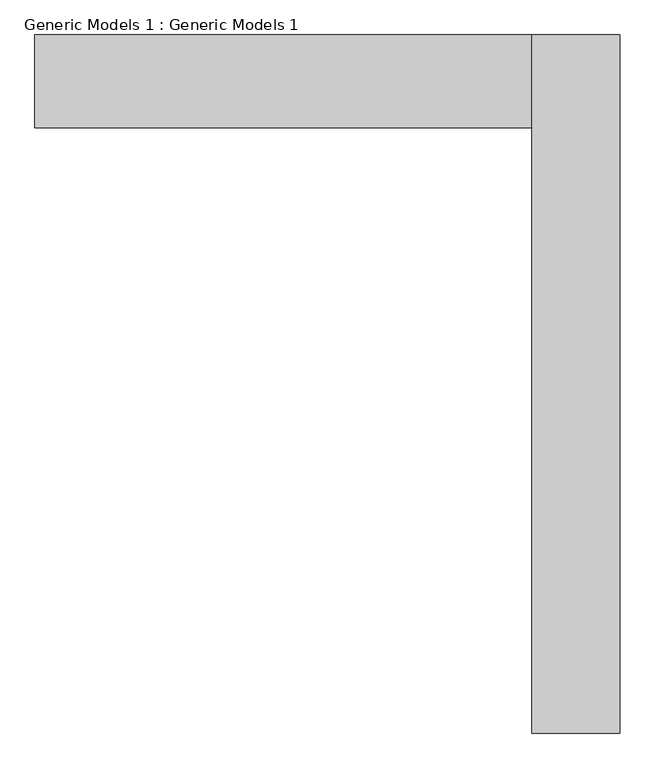
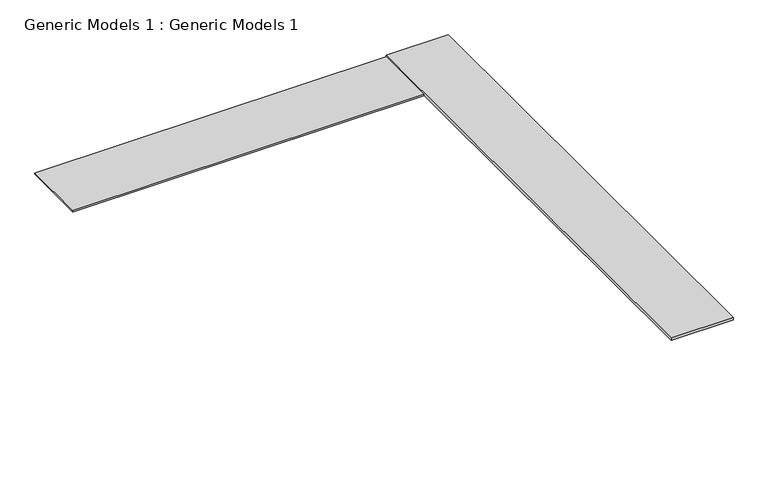
"""IFC4 building model written with IfcOpenShell, lengths in millimetres: proxy geometry, Generic Models 1 : Generic Models 1."""

from ifc_helpers import new_model, si_unit, frame, origin, place, context, project, spatial, polyline, outline, extrude, source, transform, mapped, element, save


def generic_models_1_generic_models_1_1d0d8944(model_context):
    return source(origin(), model_context, "Body", "SweptSolid", [
        extrude(outline(polyline([(14372.2188743, 18840.45), (-6031.5765858, 18840.45), (-6031.5765858, 22650.45), (14372.2188743, 22650.45), (14372.2188743, 18840.45)])), frame((0.0, 0.0, -76.2), z_axis=(0.0, 0.0, 1.0), x_axis=(1.0, 0.0, 0.0)), (0.0, 0.0, 1.0), 81.0522392),
        extrude(outline(polyline([(17971.4234142, 22650.45), (17971.4234142, -5984.104596), (14372.2188743, -5984.104596), (14372.2188743, 22650.45), (17971.4234142, 22650.45)])), frame((0.0, 0.0, -76.2), z_axis=(0.0, 0.0, 1.0), x_axis=(1.0, 0.0, 0.0)), (0.0, 0.0, 1.0), 159.7767188),
    ])


if __name__ == "__main__":
    model = new_model("IFC4")
    model_context = context("Model", 3, world=origin())
    ifc_project = project(units=[si_unit("LENGTHUNIT", "METRE", prefix="MILLI")], contexts=[model_context])
    site = spatial("IfcSite", under=ifc_project)
    building = spatial("IfcBuilding", under=site)
    placement = place(None, origin())
    generic_models_1_generic_models_1_shape = generic_models_1_generic_models_1_1d0d8944(model_context)
    element("IfcBuildingElementProxy", 1, Name="Generic Models 1 : Generic Models 1", ObjectType="Generic Models 1 : Generic Models 1", at=placement, inside=building, context=model_context, shape_type="MappedRepresentation", body=[
        mapped(generic_models_1_generic_models_1_shape, transform((0.0, 0.0, 0.0), x_axis=(1.0, 0.0, 0.0), y_axis=(0.0, 1.0, 0.0), z_axis=(0.0, 0.0, 1.0))),
    ])
    save(model, "model.ifc")
